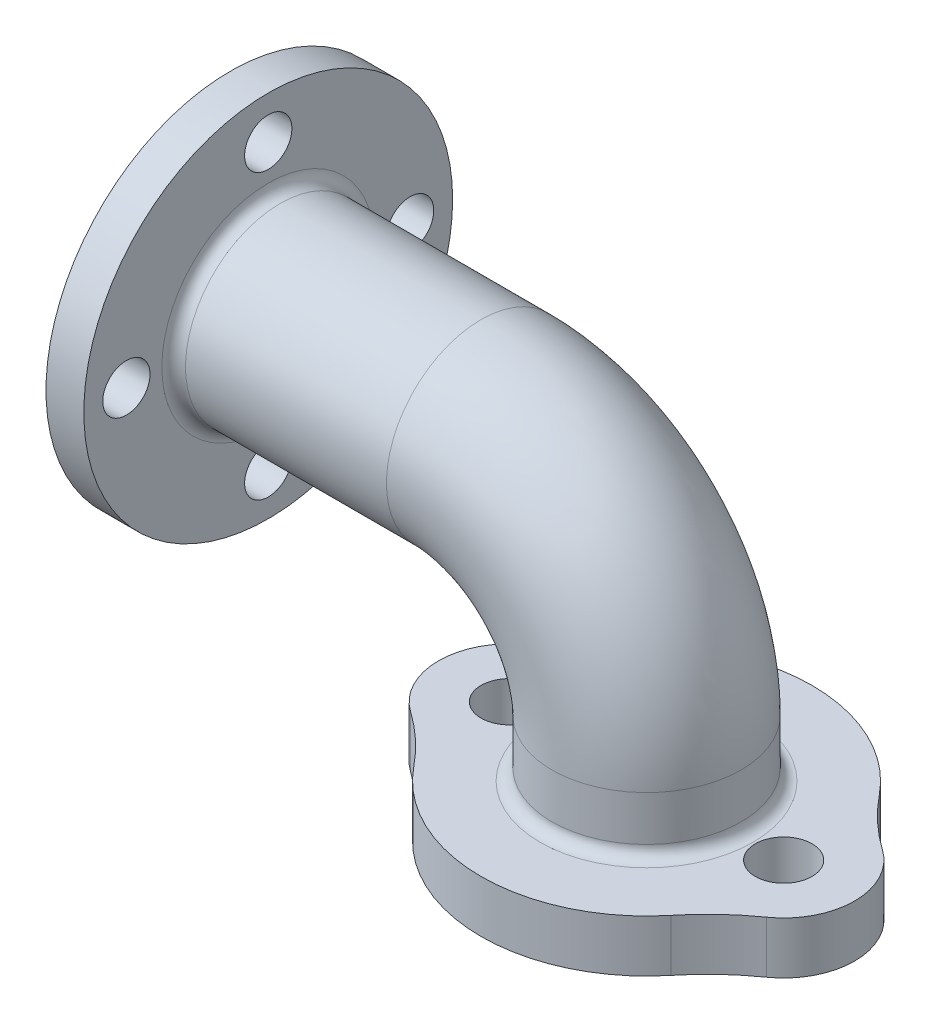
ISO-10303-21;
HEADER;
FILE_DESCRIPTION(('STEP AP214'),'2;1');
FILE_NAME('part.step','',(''),(''),'','','');
FILE_SCHEMA(('AUTOMOTIVE_DESIGN { 1 0 10303 214 1 1 1 1 }'));
ENDSEC;
DATA;
#1=APPLICATION_CONTEXT('core data for automotive mechanical design processes');
#2=APPLICATION_PROTOCOL_DEFINITION('international standard','automotive_design',2000,#1);
#3=PRODUCT_CONTEXT('',#1,'mechanical');
#4=PRODUCT('Part','Part','',(#3));
#5=PRODUCT_RELATED_PRODUCT_CATEGORY('part','',(#4));
#6=PRODUCT_DEFINITION_FORMATION('','',#4);
#7=PRODUCT_DEFINITION_CONTEXT('part definition',#1,'design');
#8=PRODUCT_DEFINITION('design','',#6,#7);
#9=PRODUCT_DEFINITION_SHAPE('','',#8);
#10=(LENGTH_UNIT() NAMED_UNIT(*) SI_UNIT(.MILLI.,.METRE.));
#11=(NAMED_UNIT(*) PLANE_ANGLE_UNIT() SI_UNIT($,.RADIAN.));
#12=(NAMED_UNIT(*) SI_UNIT($,.STERADIAN.) SOLID_ANGLE_UNIT());
#13=UNCERTAINTY_MEASURE_WITH_UNIT(LENGTH_MEASURE(1.E-05),#10,'distance_accuracy_value','');
#14=(GEOMETRIC_REPRESENTATION_CONTEXT(3) GLOBAL_UNCERTAINTY_ASSIGNED_CONTEXT((#13)) GLOBAL_UNIT_ASSIGNED_CONTEXT((#10,
#11,#12)) REPRESENTATION_CONTEXT('',''));
#15=CARTESIAN_POINT('',(0.,0.,0.));
#16=DIRECTION('',(0.,0.,1.));
#17=DIRECTION('',(1.,0.,0.));
#18=AXIS2_PLACEMENT_3D('',#15,#16,#17);
#19=CARTESIAN_POINT('',(0.,0.,0.));
#20=DIRECTION('',(1.,0.,0.));
#21=DIRECTION('',(0.,1.,0.));
#22=AXIS2_PLACEMENT_3D('',#19,#20,#21);
#23=CYLINDRICAL_SURFACE('',#22,20.);
#24=CARTESIAN_POINT('',(10.5,0.,0.));
#25=DIRECTION('',(1.,0.,0.));
#26=DIRECTION('',(0.,0.,-1.));
#27=AXIS2_PLACEMENT_3D('',#24,#25,#26);
#28=CIRCLE('',#27,20.);
#29=CARTESIAN_POINT('',(10.5,0.,-20.));
#30=VERTEX_POINT('',#29);
#31=EDGE_CURVE('E11',#30,#30,#28,.T.);
#32=ORIENTED_EDGE('',*,*,#31,.T.);
#33=EDGE_LOOP('',(#32));
#34=FACE_BOUND('',#33,.T.);
#35=CARTESIAN_POINT('',(53.,0.,0.));
#36=DIRECTION('',(1.,0.,0.));
#37=DIRECTION('',(0.,0.,-1.));
#38=AXIS2_PLACEMENT_3D('',#35,#36,#37);
#39=CIRCLE('',#38,20.);
#40=CARTESIAN_POINT('',(53.,20.,0.));
#41=VERTEX_POINT('',#40);
#42=EDGE_CURVE('E205',#41,#41,#39,.T.);
#43=ORIENTED_EDGE('',*,*,#42,.F.);
#44=EDGE_LOOP('',(#43));
#45=FACE_BOUND('',#44,.T.);
#46=ADVANCED_FACE('F41',(#34,#45),#23,.T.);
#47=CARTESIAN_POINT('',(53.,-35.,0.));
#48=DIRECTION('',(0.,0.,-1.));
#49=DIRECTION('',(-1.,0.,0.));
#50=AXIS2_PLACEMENT_3D('',#47,#48,#49);
#51=TOROIDAL_SURFACE('',#50,35.,20.);
#52=CARTESIAN_POINT('',(88.,-35.,0.));
#53=DIRECTION('',(0.,-1.,0.));
#54=DIRECTION('',(0.,0.,-1.));
#55=AXIS2_PLACEMENT_3D('',#52,#53,#54);
#56=CIRCLE('',#55,20.);
#57=CARTESIAN_POINT('',(108.,-35.,0.));
#58=VERTEX_POINT('',#57);
#59=EDGE_CURVE('E207',#58,#58,#56,.T.);
#60=CARTESIAN_POINT('',(53.,-35.,0.));
#61=DIRECTION('',(0.,0.,-1.));
#62=DIRECTION('',(-1.,0.,0.));
#63=AXIS2_PLACEMENT_3D('',#60,#61,#62);
#64=CIRCLE('',#63,55.);
#65=EDGE_CURVE('',#41,#58,#64,.T.);
#66=ORIENTED_EDGE('',*,*,#42,.T.);
#67=ORIENTED_EDGE('',*,*,#59,.F.);
#68=ORIENTED_EDGE('',*,*,#65,.T.);
#69=ORIENTED_EDGE('',*,*,#65,.F.);
#70=EDGE_LOOP('',(#66,#68,#67,#69));
#71=FACE_BOUND('',#70,.T.);
#72=ADVANCED_FACE('F271',(#71),#51,.T.);
#73=CARTESIAN_POINT('',(88.,-35.,0.));
#74=DIRECTION('',(0.,-1.,0.));
#75=DIRECTION('',(0.,0.,-1.));
#76=AXIS2_PLACEMENT_3D('',#73,#74,#75);
#77=CYLINDRICAL_SURFACE('',#76,20.);
#78=CARTESIAN_POINT('',(88.,-44.5,0.));
#79=DIRECTION('',(0.,1.,0.));
#80=DIRECTION('',(-1.,0.,0.));
#81=AXIS2_PLACEMENT_3D('',#78,#79,#80);
#82=CIRCLE('',#81,20.);
#83=CARTESIAN_POINT('',(68.,-44.5,0.));
#84=VERTEX_POINT('',#83);
#85=EDGE_CURVE('E223',#84,#84,#82,.T.);
#86=ORIENTED_EDGE('',*,*,#85,.T.);
#87=EDGE_LOOP('',(#86));
#88=FACE_BOUND('',#87,.T.);
#89=ORIENTED_EDGE('',*,*,#59,.T.);
#90=EDGE_LOOP('',(#89));
#91=FACE_BOUND('',#90,.T.);
#92=ADVANCED_FACE('F270',(#88,#91),#77,.T.);
#93=CARTESIAN_POINT('',(0.,0.,0.));
#94=DIRECTION('',(1.,0.,0.));
#95=DIRECTION('',(0.,0.,-1.));
#96=AXIS2_PLACEMENT_3D('',#93,#94,#95);
#97=PLANE('',#96);
#98=CARTESIAN_POINT('',(0.,30.,0.));
#99=DIRECTION('',(-1.,0.,0.));
#100=DIRECTION('',(0.,0.,1.));
#101=AXIS2_PLACEMENT_3D('',#98,#99,#100);
#102=CIRCLE('',#101,5.);
#103=CARTESIAN_POINT('',(0.,30.,5.));
#104=VERTEX_POINT('',#103);
#105=EDGE_CURVE('E172',#104,#104,#102,.T.);
#106=ORIENTED_EDGE('',*,*,#105,.F.);
#107=EDGE_LOOP('',(#106));
#108=FACE_BOUND('',#107,.T.);
#109=CARTESIAN_POINT('',(0.,8.47140372315957E-13,30.0000000000008));
#110=DIRECTION('',(-1.,0.,0.));
#111=DIRECTION('',(0.,0.,1.));
#112=AXIS2_PLACEMENT_3D('',#109,#110,#111);
#113=CIRCLE('',#112,5.00000000000066);
#114=CARTESIAN_POINT('',(0.,8.47140372315957E-13,35.0000000000015));
#115=VERTEX_POINT('',#114);
#116=EDGE_CURVE('E185',#115,#115,#113,.T.);
#117=ORIENTED_EDGE('',*,*,#116,.F.);
#118=EDGE_LOOP('',(#117));
#119=FACE_BOUND('',#118,.T.);
#120=CARTESIAN_POINT('',(0.,-30.,1.69428074463191E-12));
#121=DIRECTION('',(-1.,0.,0.));
#122=DIRECTION('',(0.,0.,1.));
#123=AXIS2_PLACEMENT_3D('',#120,#121,#122);
#124=CIRCLE('',#123,5.00000000000182);
#125=CARTESIAN_POINT('',(0.,-30.,5.00000000000351));
#126=VERTEX_POINT('',#125);
#127=EDGE_CURVE('E191',#126,#126,#124,.T.);
#128=ORIENTED_EDGE('',*,*,#127,.F.);
#129=EDGE_LOOP('',(#128));
#130=FACE_BOUND('',#129,.T.);
#131=CARTESIAN_POINT('',(0.,-8.50814312713399E-13,-29.9999999999992));
#132=DIRECTION('',(-1.,0.,0.));
#133=DIRECTION('',(0.,0.,1.));
#134=AXIS2_PLACEMENT_3D('',#131,#132,#133);
#135=CIRCLE('',#134,5.00000000000136);
#136=CARTESIAN_POINT('',(0.,-8.50814312713399E-13,-24.9999999999978));
#137=VERTEX_POINT('',#136);
#138=EDGE_CURVE('E193',#137,#137,#135,.T.);
#139=ORIENTED_EDGE('',*,*,#138,.F.);
#140=EDGE_LOOP('',(#139));
#141=FACE_BOUND('',#140,.T.);
#142=CARTESIAN_POINT('',(0.,0.,0.));
#143=DIRECTION('',(1.,0.,0.));
#144=DIRECTION('',(0.,0.,-1.));
#145=AXIS2_PLACEMENT_3D('',#142,#143,#144);
#146=CIRCLE('',#145,13.);
#147=CARTESIAN_POINT('',(0.,0.,-13.));
#148=VERTEX_POINT('',#147);
#149=EDGE_CURVE('E202',#148,#148,#146,.F.);
#150=ORIENTED_EDGE('',*,*,#149,.F.);
#151=EDGE_LOOP('',(#150));
#152=FACE_BOUND('',#151,.T.);
#153=CARTESIAN_POINT('',(0.,0.,0.));
#154=DIRECTION('',(1.,0.,0.));
#155=DIRECTION('',(0.,0.,-1.));
#156=AXIS2_PLACEMENT_3D('',#153,#154,#155);
#157=CIRCLE('',#156,39.);
#158=CARTESIAN_POINT('',(0.,0.,-39.));
#159=VERTEX_POINT('',#158);
#160=EDGE_CURVE('E177',#159,#159,#157,.T.);
#161=ORIENTED_EDGE('',*,*,#160,.F.);
#162=EDGE_LOOP('',(#161));
#163=FACE_BOUND('',#162,.T.);
#164=ADVANCED_FACE('F263',(#108,#119,#130,#141,#152,#163),#97,.F.);
#165=CARTESIAN_POINT('',(88.,-58.,0.));
#166=DIRECTION('',(0.,-1.,0.));
#167=DIRECTION('',(0.,0.,-1.));
#168=AXIS2_PLACEMENT_3D('',#165,#166,#167);
#169=PLANE('',#168);
#170=CARTESIAN_POINT('',(88.,-58.,0.));
#171=DIRECTION('',(0.,-1.,0.));
#172=DIRECTION('',(0.,0.,-1.));
#173=AXIS2_PLACEMENT_3D('',#170,#171,#172);
#174=CIRCLE('',#173,13.);
#175=CARTESIAN_POINT('',(88.,-58.,-13.));
#176=VERTEX_POINT('',#175);
#177=EDGE_CURVE('E214',#176,#176,#174,.F.);
#178=ORIENTED_EDGE('',*,*,#177,.T.);
#179=EDGE_LOOP('',(#178));
#180=FACE_BOUND('',#179,.T.);
#181=CARTESIAN_POINT('',(59.,-58.,0.));
#182=DIRECTION('',(0.,-1.,0.));
#183=DIRECTION('',(1.,0.,0.));
#184=AXIS2_PLACEMENT_3D('',#181,#182,#183);
#185=CIRCLE('',#184,5.99999999999999);
#186=CARTESIAN_POINT('',(65.,-58.,0.));
#187=VERTEX_POINT('',#186);
#188=EDGE_CURVE('E308',#187,#187,#185,.T.);
#189=ORIENTED_EDGE('',*,*,#188,.F.);
#190=EDGE_LOOP('',(#189));
#191=FACE_BOUND('',#190,.T.);
#192=CARTESIAN_POINT('',(117.,-58.,0.));
#193=DIRECTION('',(0.,-1.,0.));
#194=DIRECTION('',(1.,0.,0.));
#195=AXIS2_PLACEMENT_3D('',#192,#193,#194);
#196=CIRCLE('',#195,6.);
#197=CARTESIAN_POINT('',(123.,-58.,0.));
#198=VERTEX_POINT('',#197);
#199=EDGE_CURVE('E301',#198,#198,#196,.T.);
#200=ORIENTED_EDGE('',*,*,#199,.F.);
#201=EDGE_LOOP('',(#200));
#202=FACE_BOUND('',#201,.T.);
#203=CARTESIAN_POINT('',(155.603448275862,-58.,-54.76106081161));
#204=DIRECTION('',(0.,1.,0.));
#205=DIRECTION('',(-1.,0.,0.));
#206=AXIS2_PLACEMENT_3D('',#203,#204,#205);
#207=CIRCLE('',#206,52.);
#208=CARTESIAN_POINT('',(115.196789536266,-58.,-22.0303118207626));
#209=VERTEX_POINT('',#208);
#210=CARTESIAN_POINT('',(125.642563046835,-58.,-12.2599389876739));
#211=VERTEX_POINT('',#210);
#212=EDGE_CURVE('E143',#209,#211,#207,.T.);
#213=ORIENTED_EDGE('',*,*,#212,.T.);
#214=CARTESIAN_POINT('',(117.,-58.,0.));
#215=DIRECTION('',(0.,-1.,0.));
#216=DIRECTION('',(1.,0.,0.));
#217=AXIS2_PLACEMENT_3D('',#214,#215,#216);
#218=CIRCLE('',#217,15.);
#219=CARTESIAN_POINT('',(125.642563046835,-58.,12.2599389876739));
#220=VERTEX_POINT('',#219);
#221=EDGE_CURVE('E145',#211,#220,#218,.T.);
#222=ORIENTED_EDGE('',*,*,#221,.T.);
#223=CARTESIAN_POINT('',(155.603448275862,-58.,54.76106081161));
#224=DIRECTION('',(0.,1.,0.));
#225=DIRECTION('',(-1.,0.,0.));
#226=AXIS2_PLACEMENT_3D('',#223,#224,#225);
#227=CIRCLE('',#226,52.);
#228=CARTESIAN_POINT('',(115.196789536266,-58.,22.0303118207626));
#229=VERTEX_POINT('',#228);
#230=EDGE_CURVE('E146',#220,#229,#227,.T.);
#231=ORIENTED_EDGE('',*,*,#230,.T.);
#232=CARTESIAN_POINT('',(88.,-58.,0.));
#233=DIRECTION('',(0.,-1.,0.));
#234=DIRECTION('',(1.,0.,0.));
#235=AXIS2_PLACEMENT_3D('',#232,#233,#234);
#236=CIRCLE('',#235,35.);
#237=CARTESIAN_POINT('',(60.8032104637337,-58.,22.0303118207626));
#238=VERTEX_POINT('',#237);
#239=EDGE_CURVE('E151',#229,#238,#236,.T.);
#240=ORIENTED_EDGE('',*,*,#239,.T.);
#241=CARTESIAN_POINT('',(20.396551724138,-58.,54.76106081161));
#242=DIRECTION('',(0.,1.,0.));
#243=DIRECTION('',(-1.,0.,0.));
#244=AXIS2_PLACEMENT_3D('',#241,#242,#243);
#245=CIRCLE('',#244,52.);
#246=CARTESIAN_POINT('',(50.3574369531652,-58.,12.2599389876739));
#247=VERTEX_POINT('',#246);
#248=EDGE_CURVE('E152',#238,#247,#245,.T.);
#249=ORIENTED_EDGE('',*,*,#248,.T.);
#250=CARTESIAN_POINT('',(59.,-58.,0.));
#251=DIRECTION('',(0.,-1.,0.));
#252=DIRECTION('',(1.,0.,0.));
#253=AXIS2_PLACEMENT_3D('',#250,#251,#252);
#254=CIRCLE('',#253,15.);
#255=CARTESIAN_POINT('',(50.3574369531652,-58.,-12.2599389876739));
#256=VERTEX_POINT('',#255);
#257=EDGE_CURVE('E160',#247,#256,#254,.T.);
#258=ORIENTED_EDGE('',*,*,#257,.T.);
#259=CARTESIAN_POINT('',(20.396551724138,-58.,-54.76106081161));
#260=DIRECTION('',(0.,1.,0.));
#261=DIRECTION('',(1.,0.,0.));
#262=AXIS2_PLACEMENT_3D('',#259,#260,#261);
#263=CIRCLE('',#262,52.);
#264=CARTESIAN_POINT('',(60.8032104637336,-58.,-22.0303118207626));
#265=VERTEX_POINT('',#264);
#266=EDGE_CURVE('E116',#256,#265,#263,.T.);
#267=ORIENTED_EDGE('',*,*,#266,.T.);
#268=CARTESIAN_POINT('',(88.,-58.,0.));
#269=DIRECTION('',(0.,-1.,0.));
#270=DIRECTION('',(1.,0.,0.));
#271=AXIS2_PLACEMENT_3D('',#268,#269,#270);
#272=CIRCLE('',#271,35.);
#273=EDGE_CURVE('E159',#265,#209,#272,.T.);
#274=ORIENTED_EDGE('',*,*,#273,.T.);
#275=EDGE_LOOP('',(#213,#222,#231,#240,#249,#258,#267,#274));
#276=FACE_BOUND('',#275,.T.);
#277=ADVANCED_FACE('F261',(#180,#191,#202,#276),#169,.T.);
#278=CARTESIAN_POINT('',(0.,0.,0.));
#279=DIRECTION('',(1.,0.,0.));
#280=DIRECTION('',(0.,1.,0.));
#281=AXIS2_PLACEMENT_3D('',#278,#279,#280);
#282=CYLINDRICAL_SURFACE('',#281,13.);
#283=CARTESIAN_POINT('',(53.,0.,0.));
#284=DIRECTION('',(1.,0.,0.));
#285=DIRECTION('',(0.,0.,-1.));
#286=AXIS2_PLACEMENT_3D('',#283,#284,#285);
#287=CIRCLE('',#286,13.);
#288=CARTESIAN_POINT('',(53.,13.,0.));
#289=VERTEX_POINT('',#288);
#290=EDGE_CURVE('E208',#289,#289,#287,.F.);
#291=ORIENTED_EDGE('',*,*,#290,.F.);
#292=EDGE_LOOP('',(#291));
#293=FACE_BOUND('',#292,.T.);
#294=ORIENTED_EDGE('',*,*,#149,.T.);
#295=EDGE_LOOP('',(#294));
#296=FACE_BOUND('',#295,.T.);
#297=ADVANCED_FACE('F254',(#293,#296),#282,.F.);
#298=CARTESIAN_POINT('',(53.,-35.,0.));
#299=DIRECTION('',(0.,0.,-1.));
#300=DIRECTION('',(-1.,0.,0.));
#301=AXIS2_PLACEMENT_3D('',#298,#299,#300);
#302=TOROIDAL_SURFACE('',#301,35.,13.);
#303=CARTESIAN_POINT('',(88.,-35.,0.));
#304=DIRECTION('',(0.,-1.,0.));
#305=DIRECTION('',(0.,0.,-1.));
#306=AXIS2_PLACEMENT_3D('',#303,#304,#305);
#307=CIRCLE('',#306,13.);
#308=CARTESIAN_POINT('',(101.,-35.,0.));
#309=VERTEX_POINT('',#308);
#310=EDGE_CURVE('E215',#309,#309,#307,.F.);
#311=CARTESIAN_POINT('',(53.,-35.,0.));
#312=DIRECTION('',(0.,0.,-1.));
#313=DIRECTION('',(-1.,0.,0.));
#314=AXIS2_PLACEMENT_3D('',#311,#312,#313);
#315=CIRCLE('',#314,48.);
#316=EDGE_CURVE('',#289,#309,#315,.T.);
#317=ORIENTED_EDGE('',*,*,#290,.T.);
#318=ORIENTED_EDGE('',*,*,#310,.F.);
#319=ORIENTED_EDGE('',*,*,#316,.T.);
#320=ORIENTED_EDGE('',*,*,#316,.F.);
#321=EDGE_LOOP('',(#317,#319,#318,#320));
#322=FACE_BOUND('',#321,.T.);
#323=ADVANCED_FACE('F244',(#322),#302,.F.);
#324=CARTESIAN_POINT('',(88.,-35.,0.));
#325=DIRECTION('',(0.,-1.,0.));
#326=DIRECTION('',(0.,0.,-1.));
#327=AXIS2_PLACEMENT_3D('',#324,#325,#326);
#328=CYLINDRICAL_SURFACE('',#327,13.);
#329=ORIENTED_EDGE('',*,*,#310,.T.);
#330=EDGE_LOOP('',(#329));
#331=FACE_BOUND('',#330,.T.);
#332=ORIENTED_EDGE('',*,*,#177,.F.);
#333=EDGE_LOOP('',(#332));
#334=FACE_BOUND('',#333,.T.);
#335=ADVANCED_FACE('F245',(#331,#334),#328,.F.);
#336=CARTESIAN_POINT('',(8.,0.,0.));
#337=DIRECTION('',(1.,0.,0.));
#338=DIRECTION('',(0.,0.,-1.));
#339=AXIS2_PLACEMENT_3D('',#336,#337,#338);
#340=PLANE('',#339);
#341=CARTESIAN_POINT('',(8.,0.,0.));
#342=DIRECTION('',(1.,0.,0.));
#343=DIRECTION('',(0.,0.,-1.));
#344=AXIS2_PLACEMENT_3D('',#341,#342,#343);
#345=CIRCLE('',#344,22.5);
#346=CARTESIAN_POINT('',(8.,0.,-22.5));
#347=VERTEX_POINT('',#346);
#348=EDGE_CURVE('E49',#347,#347,#345,.F.);
#349=ORIENTED_EDGE('',*,*,#348,.T.);
#350=EDGE_LOOP('',(#349));
#351=FACE_BOUND('',#350,.T.);
#352=CARTESIAN_POINT('',(7.99999999999999,30.,0.));
#353=DIRECTION('',(1.,0.,0.));
#354=DIRECTION('',(0.,0.,-1.));
#355=AXIS2_PLACEMENT_3D('',#352,#353,#354);
#356=CIRCLE('',#355,5.);
#357=CARTESIAN_POINT('',(7.99999999999999,30.,-5.));
#358=VERTEX_POINT('',#357);
#359=EDGE_CURVE('E178',#358,#358,#356,.F.);
#360=ORIENTED_EDGE('',*,*,#359,.T.);
#361=EDGE_LOOP('',(#360));
#362=FACE_BOUND('',#361,.T.);
#363=CARTESIAN_POINT('',(7.99999999999999,8.47140372315957E-13,30.0000000000008));
#364=DIRECTION('',(1.,0.,0.));
#365=DIRECTION('',(0.,0.,-1.));
#366=AXIS2_PLACEMENT_3D('',#363,#364,#365);
#367=CIRCLE('',#366,5.00000000000066);
#368=CARTESIAN_POINT('',(7.99999999999999,8.47140372315957E-13,25.0000000000002));
#369=VERTEX_POINT('',#368);
#370=EDGE_CURVE('E183',#369,#369,#367,.F.);
#371=ORIENTED_EDGE('',*,*,#370,.T.);
#372=EDGE_LOOP('',(#371));
#373=FACE_BOUND('',#372,.T.);
#374=CARTESIAN_POINT('',(7.99999999999999,-30.,1.69428074463191E-12));
#375=DIRECTION('',(1.,0.,0.));
#376=DIRECTION('',(0.,0.,-1.));
#377=AXIS2_PLACEMENT_3D('',#374,#375,#376);
#378=CIRCLE('',#377,5.00000000000182);
#379=CARTESIAN_POINT('',(7.99999999999999,-30.,-5.00000000000013));
#380=VERTEX_POINT('',#379);
#381=EDGE_CURVE('E186',#380,#380,#378,.F.);
#382=ORIENTED_EDGE('',*,*,#381,.T.);
#383=EDGE_LOOP('',(#382));
#384=FACE_BOUND('',#383,.T.);
#385=CARTESIAN_POINT('',(7.99999999999999,-8.50814312713399E-13,-29.9999999999992));
#386=DIRECTION('',(1.,0.,0.));
#387=DIRECTION('',(0.,0.,-1.));
#388=AXIS2_PLACEMENT_3D('',#385,#386,#387);
#389=CIRCLE('',#388,5.00000000000136);
#390=CARTESIAN_POINT('',(7.99999999999999,-8.50814312713399E-13,-35.0000000000005));
#391=VERTEX_POINT('',#390);
#392=EDGE_CURVE('E164',#391,#391,#389,.F.);
#393=ORIENTED_EDGE('',*,*,#392,.T.);
#394=EDGE_LOOP('',(#393));
#395=FACE_BOUND('',#394,.T.);
#396=CARTESIAN_POINT('',(8.,0.,0.));
#397=DIRECTION('',(1.,0.,0.));
#398=DIRECTION('',(0.,0.,-1.));
#399=AXIS2_PLACEMENT_3D('',#396,#397,#398);
#400=CIRCLE('',#399,39.);
#401=CARTESIAN_POINT('',(8.,0.,-39.));
#402=VERTEX_POINT('',#401);
#403=EDGE_CURVE('E200',#402,#402,#400,.T.);
#404=ORIENTED_EDGE('',*,*,#403,.T.);
#405=EDGE_LOOP('',(#404));
#406=FACE_BOUND('',#405,.T.);
#407=ADVANCED_FACE('F227',(#351,#362,#373,#384,#395,#406),#340,.T.);
#408=CARTESIAN_POINT('',(8.,0.,0.));
#409=DIRECTION('',(-1.,0.,0.));
#410=DIRECTION('',(0.,0.,1.));
#411=AXIS2_PLACEMENT_3D('',#408,#409,#410);
#412=CYLINDRICAL_SURFACE('',#411,39.);
#413=ORIENTED_EDGE('',*,*,#403,.F.);
#414=EDGE_LOOP('',(#413));
#415=FACE_BOUND('',#414,.T.);
#416=ORIENTED_EDGE('',*,*,#160,.T.);
#417=EDGE_LOOP('',(#416));
#418=FACE_BOUND('',#417,.T.);
#419=ADVANCED_FACE('F252',(#415,#418),#412,.T.);
#420=CARTESIAN_POINT('',(108.001,-8.50814312713399E-13,-29.9999999999992));
#421=DIRECTION('',(-1.,0.,0.));
#422=DIRECTION('',(0.,0.,1.));
#423=AXIS2_PLACEMENT_3D('',#420,#421,#422);
#424=CYLINDRICAL_SURFACE('',#423,5.00000000000136);
#425=ORIENTED_EDGE('',*,*,#392,.F.);
#426=EDGE_LOOP('',(#425));
#427=FACE_BOUND('',#426,.T.);
#428=ORIENTED_EDGE('',*,*,#138,.T.);
#429=EDGE_LOOP('',(#428));
#430=FACE_BOUND('',#429,.T.);
#431=ADVANCED_FACE('F358',(#427,#430),#424,.F.);
#432=CARTESIAN_POINT('',(108.001,-30.,1.69428074463191E-12));
#433=DIRECTION('',(-1.,0.,0.));
#434=DIRECTION('',(0.,0.,1.));
#435=AXIS2_PLACEMENT_3D('',#432,#433,#434);
#436=CYLINDRICAL_SURFACE('',#435,5.00000000000182);
#437=ORIENTED_EDGE('',*,*,#381,.F.);
#438=EDGE_LOOP('',(#437));
#439=FACE_BOUND('',#438,.T.);
#440=ORIENTED_EDGE('',*,*,#127,.T.);
#441=EDGE_LOOP('',(#440));
#442=FACE_BOUND('',#441,.T.);
#443=ADVANCED_FACE('F352',(#439,#442),#436,.F.);
#444=CARTESIAN_POINT('',(108.001,8.47140372315957E-13,30.0000000000008));
#445=DIRECTION('',(-1.,0.,0.));
#446=DIRECTION('',(0.,0.,1.));
#447=AXIS2_PLACEMENT_3D('',#444,#445,#446);
#448=CYLINDRICAL_SURFACE('',#447,5.00000000000066);
#449=ORIENTED_EDGE('',*,*,#370,.F.);
#450=EDGE_LOOP('',(#449));
#451=FACE_BOUND('',#450,.T.);
#452=ORIENTED_EDGE('',*,*,#116,.T.);
#453=EDGE_LOOP('',(#452));
#454=FACE_BOUND('',#453,.T.);
#455=ADVANCED_FACE('F353',(#451,#454),#448,.F.);
#456=CARTESIAN_POINT('',(108.001,30.,0.));
#457=DIRECTION('',(-1.,0.,0.));
#458=DIRECTION('',(0.,0.,1.));
#459=AXIS2_PLACEMENT_3D('',#456,#457,#458);
#460=CYLINDRICAL_SURFACE('',#459,5.);
#461=ORIENTED_EDGE('',*,*,#359,.F.);
#462=EDGE_LOOP('',(#461));
#463=FACE_BOUND('',#462,.T.);
#464=ORIENTED_EDGE('',*,*,#105,.T.);
#465=EDGE_LOOP('',(#464));
#466=FACE_BOUND('',#465,.T.);
#467=ADVANCED_FACE('F334',(#463,#466),#460,.F.);
#468=CARTESIAN_POINT('',(155.603448275862,-47.,-54.76106081161));
#469=DIRECTION('',(0.,-1.,0.));
#470=DIRECTION('',(1.,0.,0.));
#471=AXIS2_PLACEMENT_3D('',#468,#469,#470);
#472=CYLINDRICAL_SURFACE('',#471,52.);
#473=ORIENTED_EDGE('',*,*,#212,.F.);
#474=DIRECTION('',(0.,-1.,0.));
#475=VECTOR('',#474,1.);
#476=CARTESIAN_POINT('',(115.196789536266,-47.,-22.0303118207626));
#477=LINE('',#476,#475);
#478=CARTESIAN_POINT('',(115.196789536266,-47.,-22.0303118207626));
#479=VERTEX_POINT('',#478);
#480=EDGE_CURVE('E59',#479,#209,#477,.T.);
#481=ORIENTED_EDGE('',*,*,#480,.F.);
#482=CARTESIAN_POINT('',(155.603448275862,-47.,-54.76106081161));
#483=DIRECTION('',(0.,1.,0.));
#484=DIRECTION('',(-1.,0.,0.));
#485=AXIS2_PLACEMENT_3D('',#482,#483,#484);
#486=CIRCLE('',#485,52.);
#487=CARTESIAN_POINT('',(125.642563046835,-47.,-12.2599389876739));
#488=VERTEX_POINT('',#487);
#489=EDGE_CURVE('E162',#479,#488,#486,.T.);
#490=ORIENTED_EDGE('',*,*,#489,.T.);
#491=DIRECTION('',(0.,-1.,0.));
#492=VECTOR('',#491,1.);
#493=CARTESIAN_POINT('',(125.642563046835,-47.,-12.2599389876739));
#494=LINE('',#493,#492);
#495=EDGE_CURVE('E97',#488,#211,#494,.T.);
#496=ORIENTED_EDGE('',*,*,#495,.T.);
#497=EDGE_LOOP('',(#473,#481,#490,#496));
#498=FACE_BOUND('',#497,.T.);
#499=ADVANCED_FACE('F322',(#498),#472,.F.);
#500=CARTESIAN_POINT('',(88.,-47.,0.));
#501=DIRECTION('',(0.,-1.,0.));
#502=DIRECTION('',(1.,0.,0.));
#503=AXIS2_PLACEMENT_3D('',#500,#501,#502);
#504=CYLINDRICAL_SURFACE('',#503,35.);
#505=ORIENTED_EDGE('',*,*,#273,.F.);
#506=DIRECTION('',(0.,-1.,0.));
#507=VECTOR('',#506,1.);
#508=CARTESIAN_POINT('',(60.8032104637336,-47.,-22.0303118207626));
#509=LINE('',#508,#507);
#510=CARTESIAN_POINT('',(60.8032104637336,-47.,-22.0303118207626));
#511=VERTEX_POINT('',#510);
#512=EDGE_CURVE('E87',#511,#265,#509,.T.);
#513=ORIENTED_EDGE('',*,*,#512,.F.);
#514=CARTESIAN_POINT('',(88.,-47.,0.));
#515=DIRECTION('',(0.,-1.,0.));
#516=DIRECTION('',(1.,0.,0.));
#517=AXIS2_PLACEMENT_3D('',#514,#515,#516);
#518=CIRCLE('',#517,35.);
#519=EDGE_CURVE('E133',#511,#479,#518,.T.);
#520=ORIENTED_EDGE('',*,*,#519,.T.);
#521=ORIENTED_EDGE('',*,*,#480,.T.);
#522=EDGE_LOOP('',(#505,#513,#520,#521));
#523=FACE_BOUND('',#522,.T.);
#524=ADVANCED_FACE('F326',(#523),#504,.T.);
#525=CARTESIAN_POINT('',(20.396551724138,-47.,-54.76106081161));
#526=DIRECTION('',(0.,-1.,0.));
#527=DIRECTION('',(1.,0.,0.));
#528=AXIS2_PLACEMENT_3D('',#525,#526,#527);
#529=CYLINDRICAL_SURFACE('',#528,52.);
#530=ORIENTED_EDGE('',*,*,#266,.F.);
#531=DIRECTION('',(0.,-1.,0.));
#532=VECTOR('',#531,1.);
#533=CARTESIAN_POINT('',(50.3574369531652,-47.,-12.2599389876739));
#534=LINE('',#533,#532);
#535=CARTESIAN_POINT('',(50.3574369531652,-47.,-12.2599389876739));
#536=VERTEX_POINT('',#535);
#537=EDGE_CURVE('E114',#536,#256,#534,.T.);
#538=ORIENTED_EDGE('',*,*,#537,.F.);
#539=CARTESIAN_POINT('',(20.396551724138,-47.,-54.76106081161));
#540=DIRECTION('',(0.,1.,0.));
#541=DIRECTION('',(1.,0.,0.));
#542=AXIS2_PLACEMENT_3D('',#539,#540,#541);
#543=CIRCLE('',#542,52.);
#544=EDGE_CURVE('E118',#536,#511,#543,.T.);
#545=ORIENTED_EDGE('',*,*,#544,.T.);
#546=ORIENTED_EDGE('',*,*,#512,.T.);
#547=EDGE_LOOP('',(#530,#538,#545,#546));
#548=FACE_BOUND('',#547,.T.);
#549=ADVANCED_FACE('F113',(#548),#529,.F.);
#550=CARTESIAN_POINT('',(59.,-47.,0.));
#551=DIRECTION('',(0.,-1.,0.));
#552=DIRECTION('',(1.,0.,0.));
#553=AXIS2_PLACEMENT_3D('',#550,#551,#552);
#554=CYLINDRICAL_SURFACE('',#553,15.);
#555=ORIENTED_EDGE('',*,*,#257,.F.);
#556=DIRECTION('',(0.,-1.,0.));
#557=VECTOR('',#556,1.);
#558=CARTESIAN_POINT('',(50.3574369531652,-47.,12.2599389876739));
#559=LINE('',#558,#557);
#560=CARTESIAN_POINT('',(50.3574369531652,-47.,12.2599389876739));
#561=VERTEX_POINT('',#560);
#562=EDGE_CURVE('E122',#561,#247,#559,.T.);
#563=ORIENTED_EDGE('',*,*,#562,.F.);
#564=CARTESIAN_POINT('',(59.,-47.,0.));
#565=DIRECTION('',(0.,-1.,0.));
#566=DIRECTION('',(1.,0.,0.));
#567=AXIS2_PLACEMENT_3D('',#564,#565,#566);
#568=CIRCLE('',#567,15.);
#569=EDGE_CURVE('E129',#561,#536,#568,.T.);
#570=ORIENTED_EDGE('',*,*,#569,.T.);
#571=ORIENTED_EDGE('',*,*,#537,.T.);
#572=EDGE_LOOP('',(#555,#563,#570,#571));
#573=FACE_BOUND('',#572,.T.);
#574=ADVANCED_FACE('F131',(#573),#554,.T.);
#575=CARTESIAN_POINT('',(20.396551724138,-47.,54.76106081161));
#576=DIRECTION('',(0.,-1.,0.));
#577=DIRECTION('',(1.,0.,0.));
#578=AXIS2_PLACEMENT_3D('',#575,#576,#577);
#579=CYLINDRICAL_SURFACE('',#578,52.);
#580=ORIENTED_EDGE('',*,*,#248,.F.);
#581=DIRECTION('',(0.,-1.,0.));
#582=VECTOR('',#581,1.);
#583=CARTESIAN_POINT('',(60.8032104637337,-47.,22.0303118207626));
#584=LINE('',#583,#582);
#585=CARTESIAN_POINT('',(60.8032104637337,-47.,22.0303118207626));
#586=VERTEX_POINT('',#585);
#587=EDGE_CURVE('E169',#586,#238,#584,.T.);
#588=ORIENTED_EDGE('',*,*,#587,.F.);
#589=CARTESIAN_POINT('',(20.396551724138,-47.,54.76106081161));
#590=DIRECTION('',(0.,1.,0.));
#591=DIRECTION('',(-1.,0.,0.));
#592=AXIS2_PLACEMENT_3D('',#589,#590,#591);
#593=CIRCLE('',#592,52.);
#594=EDGE_CURVE('E134',#586,#561,#593,.T.);
#595=ORIENTED_EDGE('',*,*,#594,.T.);
#596=ORIENTED_EDGE('',*,*,#562,.T.);
#597=EDGE_LOOP('',(#580,#588,#595,#596));
#598=FACE_BOUND('',#597,.T.);
#599=ADVANCED_FACE('F339',(#598),#579,.F.);
#600=CARTESIAN_POINT('',(88.,-47.,0.));
#601=DIRECTION('',(0.,-1.,0.));
#602=DIRECTION('',(1.,0.,0.));
#603=AXIS2_PLACEMENT_3D('',#600,#601,#602);
#604=CYLINDRICAL_SURFACE('',#603,35.);
#605=ORIENTED_EDGE('',*,*,#239,.F.);
#606=DIRECTION('',(0.,-1.,0.));
#607=VECTOR('',#606,1.);
#608=CARTESIAN_POINT('',(115.196789536266,-47.,22.0303118207626));
#609=LINE('',#608,#607);
#610=CARTESIAN_POINT('',(115.196789536266,-47.,22.0303118207626));
#611=VERTEX_POINT('',#610);
#612=EDGE_CURVE('E168',#611,#229,#609,.T.);
#613=ORIENTED_EDGE('',*,*,#612,.F.);
#614=CARTESIAN_POINT('',(88.,-47.,0.));
#615=DIRECTION('',(0.,-1.,0.));
#616=DIRECTION('',(1.,0.,0.));
#617=AXIS2_PLACEMENT_3D('',#614,#615,#616);
#618=CIRCLE('',#617,35.);
#619=EDGE_CURVE('E136',#611,#586,#618,.T.);
#620=ORIENTED_EDGE('',*,*,#619,.T.);
#621=ORIENTED_EDGE('',*,*,#587,.T.);
#622=EDGE_LOOP('',(#605,#613,#620,#621));
#623=FACE_BOUND('',#622,.T.);
#624=ADVANCED_FACE('F318',(#623),#604,.T.);
#625=CARTESIAN_POINT('',(155.603448275862,-47.,54.76106081161));
#626=DIRECTION('',(0.,-1.,0.));
#627=DIRECTION('',(1.,0.,0.));
#628=AXIS2_PLACEMENT_3D('',#625,#626,#627);
#629=CYLINDRICAL_SURFACE('',#628,52.);
#630=ORIENTED_EDGE('',*,*,#230,.F.);
#631=DIRECTION('',(0.,-1.,0.));
#632=VECTOR('',#631,1.);
#633=CARTESIAN_POINT('',(125.642563046835,-47.,12.2599389876739));
#634=LINE('',#633,#632);
#635=CARTESIAN_POINT('',(125.642563046835,-47.,12.2599389876739));
#636=VERTEX_POINT('',#635);
#637=EDGE_CURVE('E175',#636,#220,#634,.T.);
#638=ORIENTED_EDGE('',*,*,#637,.F.);
#639=CARTESIAN_POINT('',(155.603448275862,-47.,54.76106081161));
#640=DIRECTION('',(0.,1.,0.));
#641=DIRECTION('',(-1.,0.,0.));
#642=AXIS2_PLACEMENT_3D('',#639,#640,#641);
#643=CIRCLE('',#642,52.);
#644=EDGE_CURVE('E315',#636,#611,#643,.T.);
#645=ORIENTED_EDGE('',*,*,#644,.T.);
#646=ORIENTED_EDGE('',*,*,#612,.T.);
#647=EDGE_LOOP('',(#630,#638,#645,#646));
#648=FACE_BOUND('',#647,.T.);
#649=ADVANCED_FACE('F323',(#648),#629,.F.);
#650=CARTESIAN_POINT('',(117.,-47.,0.));
#651=DIRECTION('',(0.,-1.,0.));
#652=DIRECTION('',(1.,0.,0.));
#653=AXIS2_PLACEMENT_3D('',#650,#651,#652);
#654=CYLINDRICAL_SURFACE('',#653,15.);
#655=ORIENTED_EDGE('',*,*,#221,.F.);
#656=ORIENTED_EDGE('',*,*,#495,.F.);
#657=CARTESIAN_POINT('',(117.,-47.,0.));
#658=DIRECTION('',(0.,-1.,0.));
#659=DIRECTION('',(1.,0.,0.));
#660=AXIS2_PLACEMENT_3D('',#657,#658,#659);
#661=CIRCLE('',#660,15.);
#662=EDGE_CURVE('E309',#488,#636,#661,.T.);
#663=ORIENTED_EDGE('',*,*,#662,.T.);
#664=ORIENTED_EDGE('',*,*,#637,.T.);
#665=EDGE_LOOP('',(#655,#656,#663,#664));
#666=FACE_BOUND('',#665,.T.);
#667=ADVANCED_FACE('F295',(#666),#654,.T.);
#668=CARTESIAN_POINT('',(136.301724137931,-47.,-27.380530405805));
#669=DIRECTION('',(0.,1.,0.));
#670=DIRECTION('',(-1.,0.,0.));
#671=AXIS2_PLACEMENT_3D('',#668,#669,#670);
#672=PLANE('',#671);
#673=CARTESIAN_POINT('',(88.,-47.,0.));
#674=DIRECTION('',(0.,1.,0.));
#675=DIRECTION('',(-1.,0.,0.));
#676=AXIS2_PLACEMENT_3D('',#673,#674,#675);
#677=CIRCLE('',#676,22.5);
#678=CARTESIAN_POINT('',(65.5,-47.,0.));
#679=VERTEX_POINT('',#678);
#680=EDGE_CURVE('E217',#679,#679,#677,.F.);
#681=ORIENTED_EDGE('',*,*,#680,.T.);
#682=EDGE_LOOP('',(#681));
#683=FACE_BOUND('',#682,.T.);
#684=CARTESIAN_POINT('',(59.,-47.,0.));
#685=DIRECTION('',(0.,-1.,0.));
#686=DIRECTION('',(1.,0.,0.));
#687=AXIS2_PLACEMENT_3D('',#684,#685,#686);
#688=CIRCLE('',#687,5.99999999999999);
#689=CARTESIAN_POINT('',(65.,-47.,0.));
#690=VERTEX_POINT('',#689);
#691=EDGE_CURVE('E300',#690,#690,#688,.T.);
#692=ORIENTED_EDGE('',*,*,#691,.T.);
#693=EDGE_LOOP('',(#692));
#694=FACE_BOUND('',#693,.T.);
#695=CARTESIAN_POINT('',(117.,-47.,0.));
#696=DIRECTION('',(0.,-1.,0.));
#697=DIRECTION('',(1.,0.,0.));
#698=AXIS2_PLACEMENT_3D('',#695,#696,#697);
#699=CIRCLE('',#698,6.);
#700=CARTESIAN_POINT('',(123.,-47.,0.));
#701=VERTEX_POINT('',#700);
#702=EDGE_CURVE('E144',#701,#701,#699,.T.);
#703=ORIENTED_EDGE('',*,*,#702,.T.);
#704=EDGE_LOOP('',(#703));
#705=FACE_BOUND('',#704,.T.);
#706=ORIENTED_EDGE('',*,*,#489,.F.);
#707=ORIENTED_EDGE('',*,*,#519,.F.);
#708=ORIENTED_EDGE('',*,*,#544,.F.);
#709=ORIENTED_EDGE('',*,*,#569,.F.);
#710=ORIENTED_EDGE('',*,*,#594,.F.);
#711=ORIENTED_EDGE('',*,*,#619,.F.);
#712=ORIENTED_EDGE('',*,*,#644,.F.);
#713=ORIENTED_EDGE('',*,*,#662,.F.);
#714=EDGE_LOOP('',(#706,#707,#708,#709,#710,#711,#712,#713));
#715=FACE_BOUND('',#714,.T.);
#716=ADVANCED_FACE('F130',(#683,#694,#705,#715),#672,.T.);
#717=CARTESIAN_POINT('',(117.,-47.,0.));
#718=DIRECTION('',(0.,-1.,0.));
#719=DIRECTION('',(1.,0.,0.));
#720=AXIS2_PLACEMENT_3D('',#717,#718,#719);
#721=CYLINDRICAL_SURFACE('',#720,6.);
#722=ORIENTED_EDGE('',*,*,#702,.F.);
#723=EDGE_LOOP('',(#722));
#724=FACE_BOUND('',#723,.T.);
#725=ORIENTED_EDGE('',*,*,#199,.T.);
#726=EDGE_LOOP('',(#725));
#727=FACE_BOUND('',#726,.T.);
#728=ADVANCED_FACE('F292',(#724,#727),#721,.F.);
#729=CARTESIAN_POINT('',(59.,-47.,0.));
#730=DIRECTION('',(0.,-1.,0.));
#731=DIRECTION('',(1.,0.,0.));
#732=AXIS2_PLACEMENT_3D('',#729,#730,#731);
#733=CYLINDRICAL_SURFACE('',#732,5.99999999999999);
#734=ORIENTED_EDGE('',*,*,#691,.F.);
#735=EDGE_LOOP('',(#734));
#736=FACE_BOUND('',#735,.T.);
#737=ORIENTED_EDGE('',*,*,#188,.T.);
#738=EDGE_LOOP('',(#737));
#739=FACE_BOUND('',#738,.T.);
#740=ADVANCED_FACE('F239',(#736,#739),#733,.F.);
#741=CARTESIAN_POINT('',(88.,-44.5,0.));
#742=DIRECTION('',(0.,1.,0.));
#743=DIRECTION('',(-1.,0.,0.));
#744=AXIS2_PLACEMENT_3D('',#741,#742,#743);
#745=TOROIDAL_SURFACE('',#744,22.5,2.5);
#746=ORIENTED_EDGE('',*,*,#85,.F.);
#747=EDGE_LOOP('',(#746));
#748=FACE_BOUND('',#747,.T.);
#749=ORIENTED_EDGE('',*,*,#680,.F.);
#750=EDGE_LOOP('',(#749));
#751=FACE_BOUND('',#750,.T.);
#752=ADVANCED_FACE('F233',(#748,#751),#745,.F.);
#753=CARTESIAN_POINT('',(10.5,0.,0.));
#754=DIRECTION('',(1.,0.,0.));
#755=DIRECTION('',(0.,0.,-1.));
#756=AXIS2_PLACEMENT_3D('',#753,#754,#755);
#757=TOROIDAL_SURFACE('',#756,22.5,2.5);
#758=ORIENTED_EDGE('',*,*,#31,.F.);
#759=EDGE_LOOP('',(#758));
#760=FACE_BOUND('',#759,.T.);
#761=ORIENTED_EDGE('',*,*,#348,.F.);
#762=EDGE_LOOP('',(#761));
#763=FACE_BOUND('',#762,.T.);
#764=ADVANCED_FACE('F43',(#760,#763),#757,.F.);
#765=CLOSED_SHELL('',(#46,#72,#92,#164,#277,#297,#323,#335,#407,#419,#431,#443,#455,#467,#499,
#524,#549,#574,#599,#624,#649,#667,#716,#728,#740,#752,#764));
#766=MANIFOLD_SOLID_BREP('B2',#765);
#767=ADVANCED_BREP_SHAPE_REPRESENTATION('',(#18,#766),#14);
#768=SHAPE_DEFINITION_REPRESENTATION(#9,#767);
ENDSEC;
END-ISO-10303-21;
